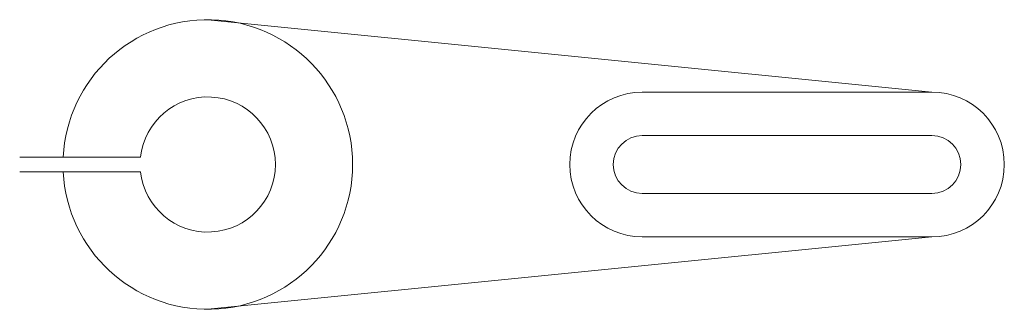
# Model space of a CAD drawing. Units: millimetres. Extents: x 2547 to 2751, y 1595 to 1655.
import ezdxf

# ---------------------------------------------------------------- set-up
doc = ezdxf.new("R2010")
doc.units = ezdxf.units.MM
doc.layers.add('M-CONS', color=8, linetype='Continuous', lineweight=18)

msp = doc.modelspace()

# ---------------------------------------------------------------- linework, layer by layer
at = {"layer": 'M-CONS'}
for p, q in [((2585.76, 1655.47), (2735.76, 1640.47)), ((2675.76, 1631.47), (2735.76, 1631.47)), ((2571.84, 1626.96), (2555.79, 1626.97)), ((2571.84, 1623.98), (2555.8, 1623.97)), ((2735.76, 1619.47), (2675.76, 1619.47)), ((2585.76, 1595.47), (2735.76, 1610.47))]:
    msp.add_line(p, q, dxfattribs=at)
msp.add_lwpolyline([(2675.76, 1640.47, 1), (2675.76, 1610.47), (2735.76, 1610.47, 1), (2735.76, 1640.47)], format="xyb", close=True, dxfattribs=at)
at = {"layer": 'M-CONS', "extrusion": (0, -1, 0)}
for elevation in [-1626.96, -1623.97]:
    msp.add_lwpolyline([(2555.8, 34), (2564.8, 34), (2564.8, 16), (2555.8, 16, -1)], format="xyb", close=True, dxfattribs=dict(at, elevation=elevation))
for centre in [(2555.8, 25, -1626.96), (2555.8, 25, -1623.97)]:
    msp.add_circle(centre, 4.5, dxfattribs=at)
at = {"layer": 'M-CONS'}
for centre, radius, start, end in [((2585.76, 1625.47), 30, 182.8659, 177.1349), ((2585.76, 1625.47), 14, 186.118, 173.8704), ((2675.76, 1625.47), 6, 90, 270), ((2735.76, 1625.47), 6, 270, 90)]:
    msp.add_arc(centre, radius, start, end, dxfattribs=at)

doc.saveas('drawing.dxf')
